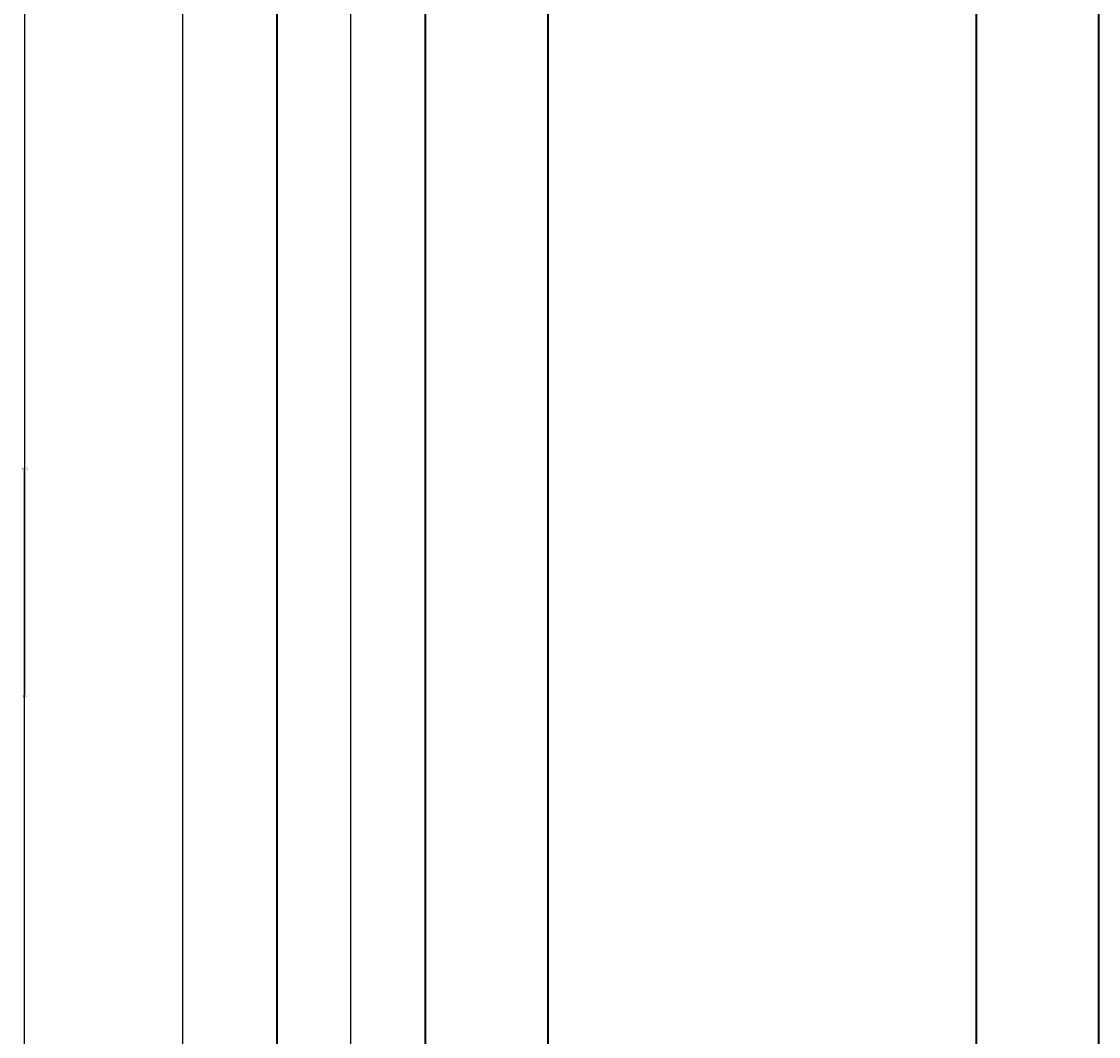
# Model space of a CAD drawing. Units: inches. Extents: x -6 to 289, y -8 to 323.
# Tile 42 of 107: x -6 to 100, y 124 to 223. Entities that reach past the tile are written whole.
import ezdxf

# ---------------------------------------------------------------- set-up
doc = ezdxf.new("R2010")
doc.units = ezdxf.units.IN
doc.header["$MEASUREMENT"] = 0
doc.layers.add('A-ANNO-DIMS', color=2, linetype='Continuous', lineweight=18)
doc.layers.add('A-ELEV', color=7, linetype='Continuous', lineweight=35)
doc.styles.get("Standard").update_dxf_attribs({"font": 'arial.ttf'})
doc.dimstyles.get("Standard").update_dxf_attribs({"dimtxt": 0.18, "dimasz": 0.18, "dimexe": 0.18, "dimexo": 0.0625, "dimgap": 0.09, "dimtad": 0, "dimtih": 1, "dimtoh": 1, "dimdec": 4, "dimzin": 0, "dimdsep": 46, "dimtxsty": 'Standard', "dimcen": 0.09, "dimadec": 0, "dimazin": 0, "dimtfac": 1, "dimtdec": 4, "dimtofl": 0, "dimtmove": 0, "dimatfit": 3, "dimfxl": 1, "dimtolj": 1, "dimtzin": 0, "dimarcsym": 0})

# ---------------------------------------------------------------- blocks, each defined once
blk = doc.blocks.new('*D19')
at = {"layer": 'A-ANNO-DIMS', "color": 0, "lineweight": -2, "transparency": 16777216}
for p, q in [((45.68, 277.04), (-5.74, 277.04)), ((-5.56, 276.86), (-5.56, 179.82)), ((-5.56, 82.42), (-5.56, 179.46)), ((45.68, 82.24), (-5.74, 82.24))]:
    blk.add_line(p, q, dxfattribs=at)
at = {"layer": 'A-ANNO-DIMS', "color": 0, "transparency": 16777216}
for points in [[(-5.59, 276.86), (-5.53, 276.86), (-5.56, 277.04)], [(-5.59, 82.42), (-5.53, 82.42), (-5.56, 82.24)]]:
    blk.add_solid(points, dxfattribs=at)
at = {"layer": 'Defpoints', "color": 0, "transparency": 16777216}
for p in [(-5.56, 277.04), (45.74, 277.04), (45.74, 82.24)]:
    blk.add_point(p, dxfattribs=at)
at = {"layer": 'A-ANNO-DIMS', "color": 0, "transparency": 16777216, "insert": (-5.56, 179.64), "char_height": 0.18, "attachment_point": 5}
blk.add_mtext('\\A1;194.8', dxfattribs=at)
blk = doc.blocks.new('*D22')
at = {"layer": 'A-ANNO-DIMS', "color": 0, "lineweight": -2, "transparency": 16777216}
for p, q in [((19.1, 307.29), (-5.74, 307.29)), ((-5.56, 307.11), (-5.56, 157.47)), ((-5.56, 7.47), (-5.56, 157.11)), ((11.91, 7.29), (-5.74, 7.29))]:
    blk.add_line(p, q, dxfattribs=at)
at = {"layer": 'A-ANNO-DIMS', "color": 0, "transparency": 16777216}
for points in [[(-5.59, 307.11), (-5.53, 307.11), (-5.56, 307.29)], [(-5.59, 7.47), (-5.53, 7.47), (-5.56, 7.29)]]:
    blk.add_solid(points, dxfattribs=at)
at = {"layer": 'Defpoints', "color": 0, "transparency": 16777216}
for p in [(19.16, 307.29), (-5.56, 7.29), (11.97, 7.29)]:
    blk.add_point(p, dxfattribs=at)
at = {"layer": 'A-ANNO-DIMS', "color": 0, "transparency": 16777216, "insert": (-5.56, 157.29), "char_height": 0.18, "attachment_point": 5}
blk.add_mtext('\\A1;300', dxfattribs=at)
blk = doc.blocks.new('*D57')
at = {"layer": 'A-ANNO-DIMS', "color": 0, "lineweight": -2, "transparency": 16777216}
for p, q in [((9.94, 68.49), (9.94, 322.97)), ((10.12, 322.79), (17.79, 322.79)), ((26.22, 322.79), (18.56, 322.79)), ((26.4, 68.49), (26.4, 322.97))]:
    blk.add_line(p, q, dxfattribs=at)
at = {"layer": 'A-ANNO-DIMS', "color": 0, "transparency": 16777216}
for points in [[(10.12, 322.82), (10.12, 322.76), (9.94, 322.79)], [(26.22, 322.82), (26.22, 322.76), (26.4, 322.79)]]:
    blk.add_solid(points, dxfattribs=at)
at = {"layer": 'Defpoints', "color": 0, "transparency": 16777216}
for p in [(26.4, 322.79), (9.94, 68.43), (26.4, 68.43)]:
    blk.add_point(p, dxfattribs=at)
at = {"layer": 'A-ANNO-DIMS', "color": 0, "transparency": 16777216, "insert": (18.17, 322.79), "char_height": 0.18, "attachment_point": 5}
blk.add_mtext('\\A1;16.46', dxfattribs=at)

msp = doc.modelspace()

# ---------------------------------------------------------------- linework, layer by layer
at = {"layer": 'A-ELEV'}
msp.add_line((19.1638, 307.2888), (19.1638, 68.4322), dxfattribs=at)
for points in [[(33.7437, 289.0427), (99.7007, 289.0427), (99.7007, 70.2425), (33.7437, 70.2425)], [(45.7437, 277.0427), (87.7007, 277.0427), (87.7007, 82.2425), (45.7437, 82.2425)]]:
    msp.add_lwpolyline(points, close=True, dxfattribs=at)

# ---------------------------------------------------------------- dimensions: what is measured, and where the dimension line sits
at = {"layer": 'A-ANNO-DIMS'}
dim = msp.add_linear_dim(base=(26.403, 322.7888), p1=(9.943, 68.4322), p2=(26.403, 68.4322), dimstyle='Standard', override={"dimdec": 2, "dimlfac": 1, "dimrnd": 0, "dimzin": 0, "dimdsep": 46, "dimlunit": 2}, dxfattribs=at)
dim.commit()
dim.dimension.update_dxf_attribs({"geometry": '*D57', "text_midpoint": (18.173, 322.7888)})
for base, p1, p2, override, picture, middle in [((-5.557, 7.2888), (19.1638, 307.2888), (11.9692, 7.2888), {"dimdec": 0, "dimlfac": 1, "dimrnd": 0, "dimzin": 0, "dimdsep": 46, "dimlunit": 2}, '*D22', (-5.557, 157.2888)), ((-5.557, 277.0427), (45.7437, 82.2425), (45.7437, 277.0427), {"dimdec": 1, "dimlfac": 1, "dimrnd": 0, "dimzin": 0, "dimdsep": 46, "dimlunit": 2}, '*D19', (-5.557, 179.6426))]:
    dim = msp.add_linear_dim(base=base, p1=p1, p2=p2, angle=90, dimstyle='Standard', override=override, dxfattribs=at)
    dim.commit()
    dim.dimension.update_dxf_attribs({"geometry": picture, "text_midpoint": middle})

doc.saveas('drawing.dxf')
